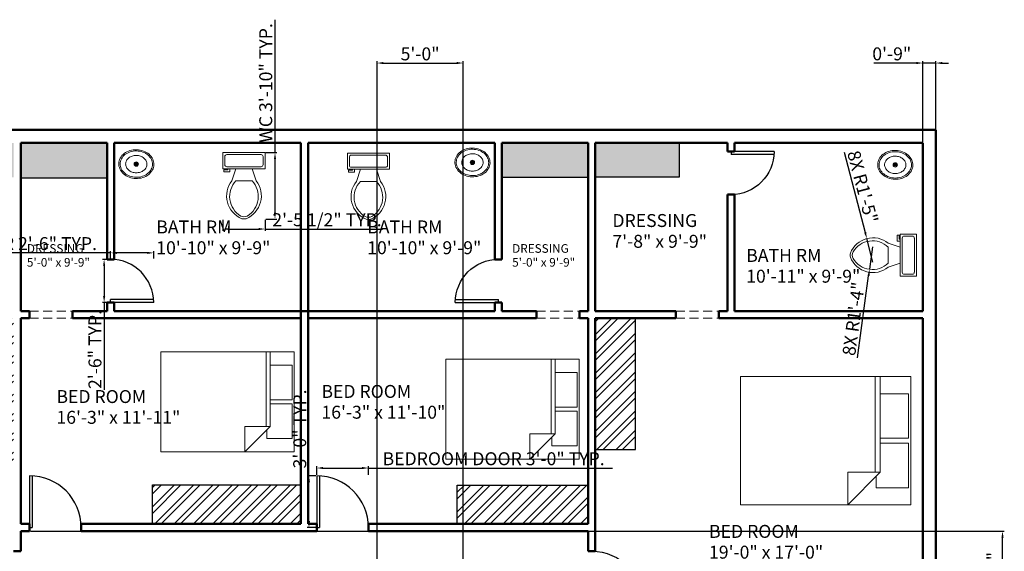
# Model space of a CAD drawing. Units: inches. Extents: x 2043 to 3102, y 1334 to 2053.
# Tile 4 of 4: x 2416 to 3102, y 1683 to 2053. Entities that reach past the tile are written whole.
import ezdxf

# ---------------------------------------------------------------- set-up
doc = ezdxf.new("R2010")
doc.units = ezdxf.units.IN
doc.linetypes.add('HIDDEN', pattern=[9.525, 6.35, -3.175])
for name, color, linetype, lineweight in [('A-ANNO-DIMS', 2, 'Continuous', 18), ('A-AREA-IDEN', 165, 'Continuous', 25), ('A-DOOR', 4, 'Continuous', 25), ('A-FLOR-CASE', 18, 'Continuous', 25), ('A-FLOR-CASE-PATT', 18, 'Continuous', 13), ('A-FLOR-FIXT', 9, 'Continuous', 20), ('A-FURN', 8, 'Continuous', 18), ('A-WALL', 7, 'Continuous', 50), ('A-WALL-OVHD', 11, 'HIDDEN', 18)]:
    doc.layers.add(name, color=color, linetype=linetype, lineweight=lineweight)
doc.styles.get("Standard").update_dxf_attribs({"font": 'arial.ttf'})
doc.dimstyles.new('ISO-25', dxfattribs={"dimtxt": 9, "dimasz": 4.5, "dimexe": 1.25, "dimexo": 0.625, "dimtad": 1, "dimdec": 0, "dimlunit": 3, "dimtxsty": 'Standard', "dimcen": 2.5, "dimadec": 0, "dimazin": 0, "dimtfac": 1, "dimtdec": 0, "dimtmove": 0, "dimatfit": 3, "dimfxl": 1, "dimarcsym": 0})

# ---------------------------------------------------------------- blocks, each defined once
blk = doc.blocks.new('Bed - Queen')
for p, q in [((0, -80.00003), (0, 0)), ((0, 0), (59.99999, 0)), ((59.99999, 0), (59.99999, -80.00003)), ((7.99999, -1.2), (28.79998, -1.2)), ((7.99999, -14.4), (7.99999, -1.2)), ((28.79998, -1.2), (28.79998, -14.4)), ((31.19999, -1.2), (51.99999, -1.2)), ((31.19999, -14.4), (31.19999, -1.2)), ((51.99999, -1.2), (51.99999, -16.4)), ((0, -14.4), (44.8, -14.4)), ((44.8, -16.8), (0, -16.8)), ((59.99999, -29.6), (44.8, -14.4)), ((44.8, -14.4), (44.8, -29.6)), ((51.99999, -16.4), (46.79936, -16.4)), ((44.8, -29.6), (59.99999, -29.6)), ((59.99999, -80.00003), (0, -80.00003))]:
    blk.add_line(p, q)
blk = doc.blocks.new('Toilet - top')
for p, q in [((9.5, -6), (9.5, -2)), ((-10, -8.5), (-8, -8.5)), ((-10, -9.5), (-10, -8.5)), ((-7, -9.5), (-10, -9.5)), ((-8, -8.5), (-8, -8)), ((-7, -8), (-7, -9.5)), ((-4, -8), (-6, -14)), ((4, -8), (6, -14)), ((4, -14), (-4, -14))]:
    blk.add_line(p, q)
blk.add_lwpolyline([(10.5, -8), (10.5, 0), (-10.5, 0), (-10.5, -8)], close=True)
for points in [[(-9.5, -2), (-9.5, -6)], [(8.5, -1), (-8.5, -1)], [(-8.5, -7), (8.5, -7)]]:
    blk.add_lwpolyline(points)
for centre, radius, start, end in [((-8.62, -1.88), 0.884, 81.8699, 188.1301), ((8.62, -1.88), 0.884, 351.8699, 98.1301), ((-8.62, -6.12), 0.884, 171.8699, 278.1301), ((8.62, -6.12), 0.884, 261.8699, 8.1301), ((3.52, -21.58), 12.17, 141.4691, 247.9714), ((4.2, -21.82), 11.33, 136.3677, 238.9468), ((-3.52, -21.58), 12.17, 292.0284, 38.5307), ((-4.2, -21.82), 11.33, 301.053, 43.6321), ((0, -27.88), 4, 245.7318, 294.2682), ((0, -29), 4, 254.8605, 285.1395)]:
    blk.add_arc(centre, radius, start, end)
blk = doc.blocks.new('Sink - Oval top')
for p, q in [((-1, 0), (1, 0)), ((0, 1), (0, -1))]:
    blk.add_line(p, q)
for points in [[(-12.23, 0.39, 0.117634), (-11.46, -3.36, 0.104469), (-8.88, -6.8, 0.090016), (-5.08, -9.07, 0.08192), (-0.32, -10.02, 0.08192), (4.49, -9.38, 0.090016), (8.42, -7.36, 0.104469), (11.22, -4.09, 0.117634), (12.23, -0.39, 0.117634), (11.46, 3.36, 0.104469), (8.88, 6.8, 0.090016), (5.08, 9.07, 0.08192), (0.32, 10.02, 0.08192), (-4.49, 9.38, 0.090016), (-8.42, 7.36, 0.104469), (-11.22, 4.09, 0.117634)], [(-11.29, 0.16, 0.118622), (-10.52, -3.25, 0.104678), (-8.07, -6.36, 0.089562), (-4.54, -8.37, 0.081185), (-0.13, -9.15, 0.081185), (4.3, -8.49, 0.089562), (7.89, -6.58, 0.104678), (10.42, -3.55, 0.118622), (11.29, -0.16, 0.118622), (10.52, 3.25, 0.104678), (8.07, 6.36, 0.089562), (4.54, 8.37, 0.081185), (0.13, 9.15, 0.081185), (-4.3, 8.49, 0.089562), (-7.89, 6.58, 0.104678), (-10.42, 3.55, 0.118622)], [(-7.42, 0.08, 0.118283), (-6.91, -2.17, 0.104607), (-5.29, -4.21, 0.089718), (-2.97, -5.53, 0.081436), (-0.07, -6.04, 0.081436), (2.84, -5.59, 0.089718), (5.2, -4.33, 0.104607), (6.86, -2.32, 0.118283), (7.42, -0.08, 0.118283), (6.91, 2.17, 0.104607), (5.29, 4.21, 0.089718), (2.97, 5.53, 0.081436), (0.07, 6.04, 0.081436), (-2.84, 5.59, 0.089718), (-5.2, 4.33, 0.104607), (-6.86, 2.32, 0.118283)]]:
    blk.add_lwpolyline(points, format="xyb", close=True)
for radius in [1.5, 1]:
    blk.add_circle((0, 0), radius)
blk = doc.blocks.new('DOOR-SWING-30IN')
for p, q in [((0, 30), (30, 30)), ((0, 28), (30, 28)), ((30, 30), (30, 28))]:
    blk.add_line(p, q)
blk.add_arc((30, 30), 30, 180, 270)
blk = doc.blocks.new('DOOR-SWING-36IN')
for p, q in [((0, 36), (0, 0)), ((2, 36), (2, 0)), ((0, 0), (2, 0))]:
    blk.add_line(p, q)
blk.add_arc((0, 0), 36, 0, 90)
blk = doc.blocks.new('*D32')
at = {"layer": 'A-ANNO-DIMS', "color": 0, "lineweight": -2, "transparency": 16777216}
for p, q in [((2594.17, 1960.48), (2594.17, 2052.89)), ((2587.87, 1960.48), (2595.42, 1960.48)), ((2594.17, 1918.77), (2594.17, 1955.98)), ((2587.87, 1914.27), (2595.42, 1914.27))]:
    blk.add_line(p, q, dxfattribs=at)
at = {"layer": 'A-ANNO-DIMS', "color": 0, "transparency": 16777216}
for points in [[(2593.42, 1955.98), (2594.92, 1955.98), (2594.17, 1960.48)], [(2593.42, 1918.77), (2594.92, 1918.77), (2594.17, 1914.27)]]:
    blk.add_solid(points, dxfattribs=at)
at = {"layer": 'Defpoints', "color": 0, "transparency": 16777216}
for p in [(2587.24, 1960.48), (2594.17, 1960.48), (2587.24, 1914.27)]:
    blk.add_point(p, dxfattribs=at)
at = {"layer": 'A-ANNO-DIMS', "color": 0, "transparency": 16777216, "insert": (2588.89, 2008.93), "char_height": 9, "attachment_point": 5, "rotation": 90}
blk.add_mtext('WC 3\'-10" TYP.', dxfattribs=at)
blk = doc.blocks.new('*D33')
at = {"layer": 'A-ANNO-DIMS', "color": 0, "lineweight": -2, "transparency": 16777216}
for p, q in [((2557.88, 1913.65), (2557.88, 1906.09)), ((2587.24, 1913.65), (2587.24, 1906.09)), ((2562.38, 1907.34), (2582.74, 1907.34)), ((2587.24, 1907.34), (2668.98, 1907.34))]:
    blk.add_line(p, q, dxfattribs=at)
at = {"layer": 'A-ANNO-DIMS', "color": 0, "transparency": 16777216}
for points in [[(2562.38, 1908.09), (2562.38, 1906.59), (2557.88, 1907.34)], [(2582.74, 1908.09), (2582.74, 1906.59), (2587.24, 1907.34)]]:
    blk.add_solid(points, dxfattribs=at)
at = {"layer": 'Defpoints', "color": 0, "transparency": 16777216}
for p in [(2557.88, 1914.27), (2587.24, 1914.27), (2587.24, 1907.34)]:
    blk.add_point(p, dxfattribs=at)
at = {"layer": 'A-ANNO-DIMS', "color": 0, "transparency": 16777216, "insert": (2630.36, 1912.62), "char_height": 9, "attachment_point": 5}
blk.add_mtext('2\'-5 1/2" TYP.', dxfattribs=at)
blk = doc.blocks.new('*D34')
at = {"layer": 'A-ANNO-DIMS', "color": 0, "lineweight": -2, "transparency": 16777216}
for p, q in [((2479.69, 1890.75), (2314.95, 1890.75)), ((2479.69, 1886.88), (2479.69, 1892)), ((2505.19, 1890.75), (2484.19, 1890.75)), ((2509.69, 1886.88), (2509.69, 1892))]:
    blk.add_line(p, q, dxfattribs=at)
at = {"layer": 'A-ANNO-DIMS', "color": 0, "transparency": 16777216}
for points in [[(2484.19, 1891.5), (2484.19, 1890), (2479.69, 1890.75)], [(2505.19, 1891.5), (2505.19, 1890), (2509.69, 1890.75)]]:
    blk.add_solid(points, dxfattribs=at)
at = {"layer": 'Defpoints', "color": 0, "transparency": 16777216}
for p in [(2479.69, 1890.75), (2479.69, 1886.25), (2509.69, 1886.25)]:
    blk.add_point(p, dxfattribs=at)
at = {"layer": 'A-ANNO-DIMS', "color": 0, "transparency": 16777216, "insert": (2395.07, 1896.04), "char_height": 9, "attachment_point": 5}
blk.add_mtext('INTERIOR DOOR 2\'-6" TYP.', dxfattribs=at)
blk = doc.blocks.new('*D35')
at = {"layer": 'A-ANNO-DIMS', "color": 0, "lineweight": -2, "transparency": 16777216}
for p, q in [((2479.06, 1886.25), (2473.94, 1886.25)), ((2475.19, 1881.75), (2475.19, 1860.75)), ((2479.06, 1856.25), (2473.94, 1856.25)), ((2475.19, 1856.25), (2475.19, 1795.49))]:
    blk.add_line(p, q, dxfattribs=at)
at = {"layer": 'A-ANNO-DIMS', "color": 0, "transparency": 16777216}
for points in [[(2474.44, 1881.75), (2475.94, 1881.75), (2475.19, 1886.25)], [(2474.44, 1860.75), (2475.94, 1860.75), (2475.19, 1856.25)]]:
    blk.add_solid(points, dxfattribs=at)
at = {"layer": 'Defpoints', "color": 0, "transparency": 16777216}
for p in [(2479.69, 1886.25), (2475.19, 1856.25), (2479.69, 1856.25)]:
    blk.add_point(p, dxfattribs=at)
at = {"layer": 'A-ANNO-DIMS', "color": 0, "transparency": 16777216, "insert": (2469.97, 1823.62), "char_height": 9, "attachment_point": 5, "rotation": 90}
blk.add_mtext('2\'-6" TYP.', dxfattribs=at)
blk = doc.blocks.new('*D36')
at = {"layer": 'A-ANNO-DIMS', "color": 0, "lineweight": -2, "transparency": 16777216}
for p, q in [((2623.19, 1736.38), (2623.19, 1742.4)), ((2659.19, 1736.38), (2659.19, 1742.4)), ((2627.69, 1741.15), (2654.69, 1741.15)), ((2659.19, 1741.15), (2829.07, 1741.15))]:
    blk.add_line(p, q, dxfattribs=at)
at = {"layer": 'A-ANNO-DIMS', "color": 0, "transparency": 16777216}
for points in [[(2627.69, 1741.9), (2627.69, 1740.4), (2623.19, 1741.15)], [(2654.69, 1741.9), (2654.69, 1740.4), (2659.19, 1741.15)]]:
    blk.add_solid(points, dxfattribs=at)
at = {"layer": 'Defpoints', "color": 0, "transparency": 16777216}
for p in [(2623.19, 1735.75), (2659.19, 1741.15), (2659.19, 1735.75)]:
    blk.add_point(p, dxfattribs=at)
at = {"layer": 'A-ANNO-DIMS', "color": 0, "transparency": 16777216, "insert": (2746.38, 1746.44), "char_height": 9, "attachment_point": 5}
blk.add_mtext('BEDROOM DOOR 3\'-0" TYP.', dxfattribs=at)
blk = doc.blocks.new('*D37')
at = {"layer": 'A-ANNO-DIMS', "color": 0, "lineweight": -2, "transparency": 16777216}
for p, q in [((2617.79, 1735.75), (2617.79, 1796.36)), ((2622.56, 1735.75), (2616.54, 1735.75)), ((2617.79, 1704.25), (2617.79, 1731.25)), ((2622.56, 1699.75), (2616.54, 1699.75))]:
    blk.add_line(p, q, dxfattribs=at)
at = {"layer": 'A-ANNO-DIMS', "color": 0, "transparency": 16777216}
for points in [[(2617.04, 1731.25), (2618.54, 1731.25), (2617.79, 1735.75)], [(2617.04, 1704.25), (2618.54, 1704.25), (2617.79, 1699.75)]]:
    blk.add_solid(points, dxfattribs=at)
at = {"layer": 'Defpoints', "color": 0, "transparency": 16777216}
for p in [(2617.79, 1735.75), (2623.19, 1735.75), (2623.19, 1699.75)]:
    blk.add_point(p, dxfattribs=at)
at = {"layer": 'A-ANNO-DIMS', "color": 0, "transparency": 16777216, "insert": (2612.56, 1768.31), "char_height": 9, "attachment_point": 5, "rotation": 90}
blk.add_mtext('3\'-0" TYP.', dxfattribs=at)
blk = doc.blocks.new('*D60')
at = {"layer": 'A-ANNO-DIMS', "color": 0, "lineweight": -2, "transparency": 16777216}
for p, q in [((2423.81, 1697.25), (3101.95, 1697.25)), ((3100.7, 1645.75), (3100.7, 1692.75)), ((2417.81, 1641.25), (3101.95, 1641.25))]:
    blk.add_line(p, q, dxfattribs=at)
at = {"layer": 'A-ANNO-DIMS', "color": 0, "transparency": 16777216}
for points in [[(3099.95, 1692.75), (3101.45, 1692.75), (3100.7, 1697.25)], [(3099.95, 1645.75), (3101.45, 1645.75), (3100.7, 1641.25)]]:
    blk.add_solid(points, dxfattribs=at)
at = {"layer": 'Defpoints', "color": 0, "transparency": 16777216}
for p in [(2423.19, 1697.25), (3100.7, 1697.25), (2417.19, 1641.25)]:
    blk.add_point(p, dxfattribs=at)
at = {"layer": 'A-ANNO-DIMS', "color": 0, "transparency": 16777216, "insert": (3095.48, 1669.25), "char_height": 9, "attachment_point": 5, "rotation": 90}
blk.add_mtext('4\'-8"', dxfattribs=at)
blk = doc.blocks.new('*D63')
at = {"layer": 'A-ANNO-DIMS', "color": 0, "lineweight": -2, "transparency": 16777216}
for p, q in [((3040.69, 2022.76), (3011.01, 2022.76)), ((3045.19, 1967.88), (3045.19, 2024.01)), ((3054.19, 2022.76), (3045.19, 2022.76)), ((3054.19, 1976.88), (3054.19, 2024.01)), ((3058.69, 2022.76), (3063.19, 2022.76))]:
    blk.add_line(p, q, dxfattribs=at)
at = {"layer": 'A-ANNO-DIMS', "color": 0, "transparency": 16777216}
for points in [[(3040.69, 2023.51), (3040.69, 2022.01), (3045.19, 2022.76)], [(3058.69, 2023.51), (3058.69, 2022.01), (3054.19, 2022.76)]]:
    blk.add_solid(points, dxfattribs=at)
at = {"layer": 'Defpoints', "color": 0, "transparency": 16777216}
for p in [(3045.19, 2022.76), (3054.19, 1976.25), (3045.19, 1967.25)]:
    blk.add_point(p, dxfattribs=at)
at = {"layer": 'A-ANNO-DIMS', "color": 0, "transparency": 16777216, "insert": (3023.6, 2027.98), "char_height": 9, "attachment_point": 5}
blk.add_mtext('0\'-9"', dxfattribs=at)
blk = doc.blocks.new('*D67')
at = {"layer": 'A-ANNO-DIMS', "color": 0, "lineweight": -2, "transparency": 16777216}
for p, q in [((2665.19, 1641.88), (2665.19, 2024.01)), ((2669.69, 2022.76), (2720.69, 2022.76)), ((2725.19, 1641.88), (2725.19, 2024.01))]:
    blk.add_line(p, q, dxfattribs=at)
at = {"layer": 'A-ANNO-DIMS', "color": 0, "transparency": 16777216}
for points in [[(2669.69, 2023.51), (2669.69, 2022.01), (2665.19, 2022.76)], [(2720.69, 2023.51), (2720.69, 2022.01), (2725.19, 2022.76)]]:
    blk.add_solid(points, dxfattribs=at)
at = {"layer": 'Defpoints', "color": 0, "transparency": 16777216}
for p in [(2725.19, 2022.76), (2665.19, 1641.25), (2725.19, 1641.25)]:
    blk.add_point(p, dxfattribs=at)
at = {"layer": 'A-ANNO-DIMS', "color": 0, "transparency": 16777216, "insert": (2695.19, 2027.98), "char_height": 9, "attachment_point": 5}
blk.add_mtext('5\'-0"', dxfattribs=at)
blk = doc.blocks.new('*D73')
at = {"layer": 'A-ANNO-DIMS', "color": 0, "lineweight": -2, "transparency": 16777216}
for p, q in [((2990.41, 1960.78), (3005.06, 1905.04)), ((3010.52, 1884.23), (3006.2, 1900.68))]:
    blk.add_line(p, q, dxfattribs=at)
at = {"layer": 'A-ANNO-DIMS', "color": 0, "transparency": 16777216}
blk.add_solid([(3005.78, 1905.23), (3004.33, 1904.85), (3006.2, 1900.68)], dxfattribs=at)
at = {"layer": 'Defpoints', "color": 0, "transparency": 16777216}
for p in [(3006.2, 1900.68), (3010.52, 1884.23)]:
    blk.add_point(p, dxfattribs=at)
at = {"layer": 'A-ANNO-DIMS', "color": 0, "transparency": 16777216, "insert": (3002.21, 1936.41), "char_height": 9, "attachment_point": 5, "rotation": 284.72105}
blk.add_mtext('8X R1\'-5"', dxfattribs=at)
blk = doc.blocks.new('*D74')
at = {"layer": 'A-ANNO-DIMS', "color": 0, "lineweight": -2, "transparency": 16777216}
for p, q in [((3010.19, 1895.02), (3008.08, 1879.32)), ((2999.8, 1817.74), (3007.48, 1874.86))]:
    blk.add_line(p, q, dxfattribs=at)
at = {"layer": 'A-ANNO-DIMS', "color": 0, "transparency": 16777216}
blk.add_solid([(3006.74, 1874.96), (3008.23, 1874.76), (3008.08, 1879.32)], dxfattribs=at)
at = {"layer": 'Defpoints', "color": 0, "transparency": 16777216}
for p in [(3010.19, 1895.02), (3008.08, 1879.32)]:
    blk.add_point(p, dxfattribs=at)
at = {"layer": 'A-ANNO-DIMS', "color": 0, "transparency": 16777216, "insert": (2998.17, 1844.76), "char_height": 9, "attachment_point": 5, "rotation": 82.34323}
blk.add_mtext('8X R1\'-4"', dxfattribs=at)

msp = doc.modelspace()

# ---------------------------------------------------------------- hatches: boundary and pattern name
at = {"layer": 'A-FLOR-CASE-PATT'}
h = msp.add_hatch(dxfattribs=at)
h.set_pattern_fill('ANSI36', color=256)
h.paths.add_polyline_path([(2412.19, 1967.25), (2354.72, 1967.25), (2354.72, 1943.39), (2412.19, 1943.39)])
h.paths.add_polyline_path([(2477.19, 1967.25), (2417.19, 1967.25), (2417.19, 1943.04), (2477.19, 1943.04)])
h.paths.add_polyline_path([(2812.19, 1967.25), (2752.19, 1967.25), (2752.19, 1943.42), (2812.19, 1943.42)])
h.paths.add_polyline_path([(2875.74, 1967.25), (2817.19, 1967.25), (2817.19, 1943.74), (2875.74, 1943.74)])
h = msp.add_hatch(dxfattribs=at)
h.set_pattern_fill('ANSI32', color=256)
h.paths.add_polyline_path([(2412.19, 1845.25), (2384.99, 1845.25), (2384.99, 1741.79), (2412.19, 1741.79)])
h.paths.add_polyline_path([(2845.19, 1845.25), (2817.19, 1845.25), (2817.19, 1753.98), (2845.19, 1753.98)])
h = msp.add_hatch(dxfattribs=at)
h.set_pattern_fill('ANSI32', color=256)
h.paths.add_polyline_path([(2293.13, 1418.11), (2184.19, 1418.11), (2184.19, 1391.25), (2293.13, 1391.25)])
h.paths.add_polyline_path([(2812.19, 1729.23), (2721.07, 1729.23), (2721.07, 1702.25), (2812.19, 1702.25)])
h.paths.add_polyline_path([(2612.19, 1729.38), (2508.87, 1729.38), (2508.87, 1702.25), (2612.19, 1702.25)])

# ---------------------------------------------------------------- linework, layer by layer
at = {"layer": 'A-FLOR-CASE'}
for p, q in [((2417.19, 1967.25), (2417.19, 1943.04)), ((2477.19, 1967.25), (2417.19, 1967.25)), ((2477.19, 1943.04), (2477.19, 1967.25)), ((2752.19, 1967.25), (2752.19, 1943.42)), ((2812.19, 1967.25), (2752.19, 1967.25)), ((2812.19, 1943.42), (2812.19, 1967.25)), ((2817.19, 1967.25), (2817.19, 1943.74)), ((2875.74, 1943.74), (2875.74, 1967.25)), ((2417.19, 1943.04), (2477.19, 1943.04)), ((2752.19, 1943.42), (2812.19, 1943.42)), ((2817.19, 1943.74), (2875.74, 1943.74)), ((2845.19, 1753.98), (2845.19, 1845.25)), ((2817.19, 1753.98), (2845.19, 1753.98)), ((2508.87, 1702.25), (2508.87, 1729.38)), ((2508.87, 1729.38), (2612.19, 1729.38)), ((2721.07, 1702.25), (2721.07, 1729.23)), ((2721.07, 1729.23), (2812.19, 1729.23)), ((2612.19, 1702.25), (2508.87, 1702.25)), ((2812.19, 1702.25), (2721.07, 1702.25))]:
    msp.add_line(p, q, dxfattribs=at)
at = {"layer": 'A-WALL'}
for p, q in [((2175.19, 1976.25), (3054.19, 1976.25)), ((3054.19, 1976.25), (3054.19, 1382.25)), ((2417.19, 1967.25), (2417.19, 1850.25)), ((2417.19, 1967.25), (2477.19, 1967.25)), ((2477.19, 1967.25), (2477.19, 1886.25)), ((2482.19, 1967.25), (2612.19, 1967.25)), ((2482.19, 1967.25), (2482.19, 1886.25)), ((2482.19, 1967.25), (2547.19, 1967.25)), ((2612.19, 1967.25), (2612.19, 1702.25)), ((2617.19, 1967.25), (2617.19, 1702.25)), ((2617.19, 1967.25), (2747.19, 1967.25)), ((2617.19, 1967.25), (2677.69, 1967.25)), ((2747.19, 1967.25), (2747.19, 1886.25)), ((2752.19, 1967.25), (2752.19, 1886.25)), ((2752.19, 1967.25), (2812.19, 1967.25)), ((2812.19, 1967.25), (2812.19, 1850.25)), ((2817.19, 1967.25), (2817.19, 1850.25)), ((2817.19, 1967.25), (2909.19, 1967.25)), ((2909.19, 1967.25), (2909.19, 1961.25)), ((2909.19, 1961.25), (2914.19, 1961.25)), ((2914.19, 1967.25), (2914.19, 1961.25)), ((2914.19, 1967.25), (3045.19, 1967.25)), ((3045.19, 1967.25), (3045.19, 1850.25)), ((2909.19, 1931.25), (2914.19, 1931.25)), ((2909.19, 1931.25), (2909.19, 1893.75)), ((2914.19, 1931.25), (2914.19, 1893.75)), ((2909.19, 1893.75), (2909.19, 1850.25)), ((2914.19, 1893.75), (2914.19, 1850.25)), ((2477.19, 1886.25), (2482.19, 1886.25)), ((2747.19, 1886.25), (2752.19, 1886.25)), ((2477.19, 1856.25), (2482.19, 1856.25)), ((2477.19, 1856.25), (2477.19, 1850.25)), ((2482.19, 1856.25), (2482.19, 1850.25)), ((2747.19, 1856.25), (2752.19, 1856.25)), ((2747.19, 1856.25), (2747.19, 1850.25)), ((2752.19, 1856.25), (2752.19, 1850.25)), ((2417.19, 1850.25), (2423.19, 1850.25)), ((2417.19, 1845.25), (2417.19, 1702.25)), ((2417.19, 1845.25), (2423.19, 1845.25)), ((2423.19, 1850.25), (2423.19, 1845.25)), ((2453.19, 1850.25), (2453.19, 1845.25)), ((2453.19, 1850.25), (2477.19, 1850.25)), ((2453.19, 1845.25), (2612.19, 1845.25)), ((2482.19, 1850.25), (2677.69, 1850.25)), ((2482.19, 1850.25), (2547.19, 1850.25)), ((2617.19, 1850.25), (2747.19, 1850.25)), ((2617.19, 1845.25), (2688.69, 1845.25)), ((2688.69, 1845.25), (2776.19, 1845.25)), ((2752.19, 1850.25), (2776.19, 1850.25)), ((2776.19, 1850.25), (2776.19, 1845.25)), ((2806.19, 1850.25), (2806.19, 1845.25)), ((2806.19, 1850.25), (2812.19, 1850.25)), ((2806.19, 1845.25), (2812.19, 1845.25)), ((2812.19, 1845.25), (2812.19, 1702.25)), ((2817.19, 1850.25), (2873.19, 1850.25)), ((2817.19, 1845.25), (2817.19, 1683.25)), ((2817.19, 1845.25), (2873.19, 1845.25)), ((2873.19, 1850.25), (2873.19, 1845.25)), ((2903.19, 1850.25), (2903.19, 1845.25)), ((2903.19, 1850.25), (2909.19, 1850.25)), ((2903.19, 1845.25), (3045.19, 1845.25)), ((2914.19, 1850.25), (3045.19, 1850.25)), ((3045.19, 1845.25), (3045.19, 1641.25)), ((2417.19, 1702.25), (2423.19, 1702.25)), ((2423.19, 1702.25), (2423.19, 1697.25)), ((2459.19, 1702.25), (2459.19, 1697.25)), ((2459.19, 1702.25), (2612.19, 1702.25)), ((2617.19, 1702.25), (2623.19, 1702.25)), ((2623.19, 1702.25), (2623.19, 1697.25)), ((2659.19, 1702.25), (2659.19, 1697.25)), ((2659.19, 1702.25), (2812.19, 1702.25)), ((2417.19, 1697.25), (2423.19, 1697.25)), ((2417.19, 1697.25), (2417.19, 1683.25)), ((2459.19, 1697.25), (2623.19, 1697.25)), ((2659.19, 1697.25), (2812.19, 1697.25)), ((2812.19, 1697.25), (2812.19, 1683.25)), ((2412.19, 1683.25), (2417.19, 1683.25)), ((2812.19, 1683.25), (2817.19, 1683.25))]:
    msp.add_line(p, q, dxfattribs=at)
at = {"layer": 'A-WALL-OVHD'}
for p, q in [((2423.19, 1850.25), (2453.19, 1850.25)), ((2423.19, 1845.25), (2453.19, 1845.25)), ((2776.19, 1850.25), (2809.19, 1850.25)), ((2776.19, 1845.25), (2806.19, 1845.25)), ((2873.19, 1850.25), (2903.19, 1850.25)), ((2873.19, 1845.25), (2903.19, 1845.25))]:
    msp.add_line(p, q, dxfattribs=at)

# ---------------------------------------------------------------- block references
at = {"layer": 'A-DOOR', "extrusion": (0, 0, -1), "zscale": -1}
msp.add_blockref('DOOR-SWING-30IN', (-2941.69, 1931.26), dxfattribs=at)
at = {"layer": 'A-DOOR', "rotation": 180}
msp.add_blockref('DOOR-SWING-30IN', (2509.69, 1886.25), dxfattribs=at)
at = {"layer": 'A-DOOR', "extrusion": (0, 0, -1), "zscale": -1}
for name, p, rotation in [('DOOR-SWING-30IN', (-2719.69, 1886.25), 180), ('DOOR-SWING-36IN', (-2814.69, 1647.26), 90.0000000000006)]:
    msp.add_blockref(name, p, dxfattribs=dict(at, rotation=rotation))
at = {"layer": 'A-DOOR'}
for p in [(2423.19, 1699.75), (2623.19, 1699.75)]:
    msp.add_blockref('DOOR-SWING-36IN', p, dxfattribs=at)
at = {"layer": 'A-FLOR-FIXT'}
for p in [(2497.6, 1952.49), (2731.64, 1953.65), (3026.02, 1951.97)]:
    msp.add_blockref('Sink - Oval top', p, dxfattribs=at)
at = {"layer": 'A-FLOR-FIXT', "xscale": 1.398246622267437, "yscale": 1.398246622267437, "zscale": 1.398246622267437}
for p in [(2572.56, 1960.48), (2659.21, 1960.05)]:
    msp.add_blockref('Toilet - top', p, dxfattribs=at)
at = {"layer": 'A-FLOR-FIXT', "xscale": 1.398246622267437, "yscale": 1.398246622267437, "zscale": 1.398246622267437, "rotation": 270}
msp.add_blockref('Toilet - top', (3040.7, 1889.15), dxfattribs=at)
at = {"layer": 'A-FURN', "rotation": 270}
for p, xscale, yscale, zscale in [((2607.41, 1821.88), 1.159729474409778, 1.159729474409778, 1.159729474409778), ((2805.92, 1816.82), 1.159729474409778, 1.159729474409778, 1.159729474409778), ((3036.98, 1804.71), 1.485242787327834, 1.485242787327834, 1.485242787327834)]:
    msp.add_blockref('Bed - Queen', p, dxfattribs=dict(at, xscale=xscale, yscale=yscale, zscale=zscale))

# ---------------------------------------------------------------- texts
at = {"layer": 'A-AREA-IDEN'}
for s, height, p in [('BATH RM', 9, (2511.5, 1904.3)), ('BATH RM', 9, (2658.36, 1904.3)), ('DRESSING', 9, (2829.09, 1908.75)), ('10\'-10" x 9\'-9"', 9, (2511.5, 1889.84)), ('10\'-10" x 9\'-9"', 9, (2658.36, 1889.84)), ('7\'-8" x 9\'-9"', 9, (2829.09, 1894.3)), ('DRESSING', 6, (2421.42, 1890.82)), ('DRESSING', 6, (2759.29, 1890.82)), ('BATH RM', 9, (2922.24, 1884.48)), ('5\'-0" x 9\'-9"', 6, (2421.42, 1881.18)), ('5\'-0" x 9\'-9"', 6, (2759.29, 1881.18)), ('10\'-11" x 9\'-9"', 9, (2922.24, 1870.03)), ('BED ROOM ', 9, (2626.49, 1789.91)), ('BED ROOM ', 9, (2441.99, 1786.34)), ('16\'-3" x 11\'-10"', 9, (2626.49, 1775.46)), ('16\'-3" x 11\'-11"', 9, (2441.99, 1771.89)), ('BED ROOM ', 9, (2896.35, 1692.59)), ('19\'-0" x 17\'-0"', 9, (2896.35, 1678.13))]:
    msp.add_text(s, height=height, dxfattribs=at).set_placement(p)

# ---------------------------------------------------------------- dimensions: what is measured, and where the dimension line sits
at = {"layer": 'A-ANNO-DIMS'}
for base, p1, p2, angle, text, picture, middle in [((2594.17, 1960.48), (2587.24, 1914.27), (2587.24, 1960.48), 90, 'WC <> TYP.', '*D32', (2588.89, 2008.93)), ((2479.69, 1890.75), (2509.69, 1886.25), (2479.69, 1886.25), 180, 'INTERIOR DOOR <> TYP.', '*D34', (2395.07, 1896.04)), ((2475.19, 1856.25), (2479.69, 1886.25), (2479.69, 1856.25), 270, '<> TYP.', '*D35', (2469.97, 1823.62)), ((2617.79, 1735.75), (2623.19, 1699.75), (2623.19, 1735.75), 90, '<> TYP.', '*D37', (2612.56, 1768.31))]:
    dim = msp.add_linear_dim(base=base, p1=p1, p2=p2, angle=angle, text=text, dimstyle='ISO-25', override={"dimdec": 1, "dimlfac": 1, "dimrnd": 0, "dimzin": 1, "dimdsep": 46, "dimlunit": 4, "dimfrac": 2}, dxfattribs=at)
    dim.commit()
    dim.dimension.update_dxf_attribs({"geometry": picture, "text_midpoint": middle})
for base, p1, p2, picture, middle in [((2725.19, 2022.76), (2665.19, 1641.25), (2725.19, 1641.25), '*D67', (2695.19, 2027.98)), ((3045.19, 2022.76), (3054.19, 1976.25), (3045.19, 1967.25), '*D63', (3023.6, 2027.98))]:
    dim = msp.add_linear_dim(base=base, p1=p1, p2=p2, dimstyle='ISO-25', override={"dimdec": 1, "dimlfac": 1, "dimrnd": 0, "dimzin": 1, "dimdsep": 46, "dimlunit": 4, "dimfrac": 2}, dxfattribs=at)
    dim.commit()
    dim.dimension.update_dxf_attribs({"geometry": picture, "text_midpoint": middle})
for center, mpoint, picture, middle in [((3010.52, 1884.23), (3006.2, 1900.68), '*D73', (3002.21, 1936.41)), ((3010.19, 1895.02), (3008.08, 1879.32), '*D74', (2998.17, 1844.76))]:
    dim = msp.add_radius_dim(center=center, mpoint=mpoint, text='8X <>', dimstyle='ISO-25', override={"dimdec": 1, "dimlfac": 1, "dimrnd": 0, "dimzin": 1, "dimdsep": 46, "dimlunit": 4, "dimfrac": 2}, dxfattribs=at)
    dim.commit()
    dim.dimension.update_dxf_attribs({"geometry": picture, "text_midpoint": middle})
for base, p1, p2, text, picture, middle in [((2587.24, 1907.34), (2557.88, 1914.27), (2587.24, 1914.27), '<> TYP.', '*D33', (2630.36, 1912.62)), ((2659.19, 1741.15), (2623.19, 1735.75), (2659.19, 1735.75), 'BEDROOM DOOR <> TYP.', '*D36', (2746.38, 1746.44))]:
    dim = msp.add_linear_dim(base=base, p1=p1, p2=p2, text=text, dimstyle='ISO-25', override={"dimdec": 1, "dimlfac": 1, "dimrnd": 0, "dimzin": 1, "dimdsep": 46, "dimlunit": 4, "dimfrac": 2}, dxfattribs=at)
    dim.commit()
    dim.dimension.update_dxf_attribs({"geometry": picture, "text_midpoint": middle})
dim = msp.add_linear_dim(base=(3100.7, 1697.25), p1=(2417.19, 1641.25), p2=(2423.19, 1697.25), angle=90, dimstyle='ISO-25', override={"dimdec": 1, "dimlfac": 1, "dimrnd": 0, "dimzin": 1, "dimdsep": 46, "dimlunit": 4, "dimfrac": 2}, dxfattribs=at)
dim.commit()
dim.dimension.update_dxf_attribs({"geometry": '*D60', "text_midpoint": (3095.48, 1669.25)})

doc.saveas('drawing.dxf')
